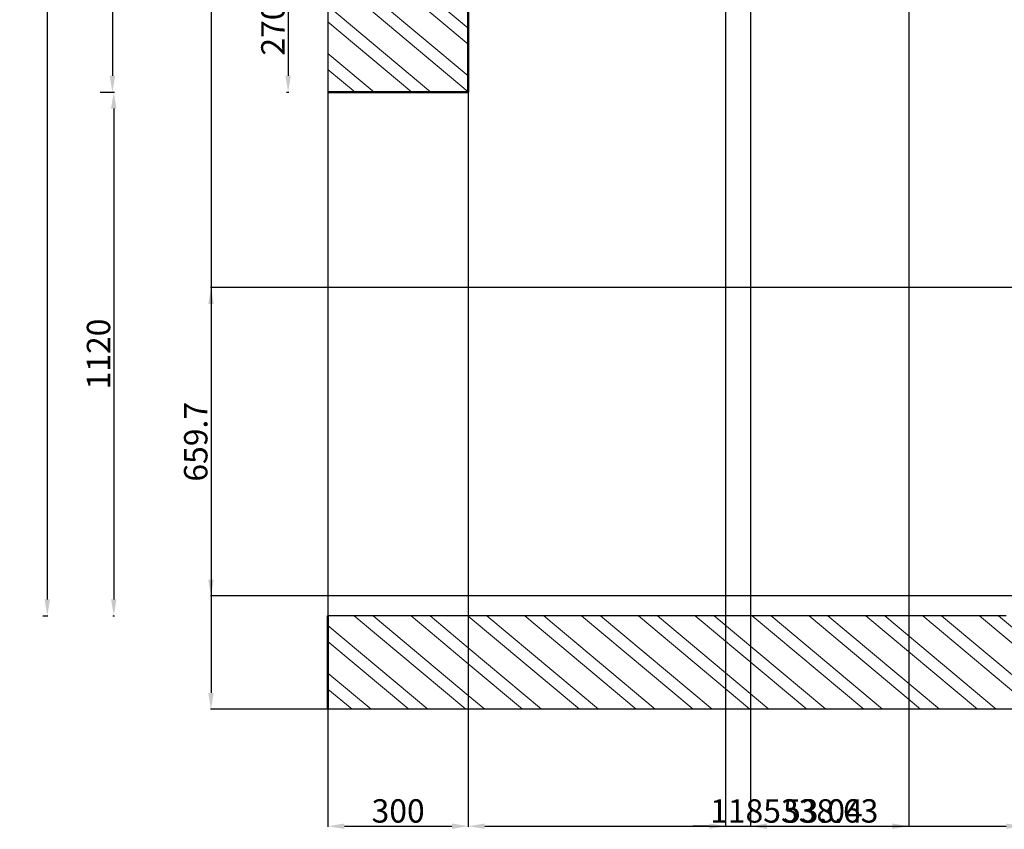
# Model space of a CAD drawing. Units: millimetres. Extents: x 407065 to 421840, y 1168257 to 1177792.
# Tile 3 of 17: x 407065 to 409170, y 1172891 to 1174623. Entities that reach past the tile are written whole.
import ezdxf

# ---------------------------------------------------------------- set-up
doc = ezdxf.new("R2010")
doc.units = ezdxf.units.MM
doc.linetypes.add('DASHED', pattern=[19.05, 12.7, -6.35])
for name, color, linetype, lineweight in [('A-ANNO-DIMS', 6, 'Continuous', 18), ('A-FURN', 3, 'Continuous', 25), ('A-FURN-HIDN', 7, 'DASHED', 18), ('A-WALL', 7, 'Continuous', 50), ('A-WALL-PATT', 8, 'Continuous', 13)]:
    doc.layers.add(name, color=color, linetype=linetype, lineweight=lineweight)
doc.styles.get("Standard").update_dxf_attribs({"font": 'arial.ttf'})
doc.dimstyles.new('ISO-25', dxfattribs={"dimtxt": 50, "dimasz": 35, "dimexe": 1.25, "dimexo": 0.625, "dimtad": 1, "dimdec": 1, "dimtxsty": 'Standard', "dimcen": 35, "dimadec": 0, "dimazin": 0, "dimtfac": 1, "dimtdec": 1, "dimtmove": 0, "dimatfit": 3, "dimfxl": 1, "dimarcsym": 0})

# ---------------------------------------------------------------- blocks, each defined once
blk = doc.blocks.new('*D43')
at = {"layer": 'A-ANNO-DIMS', "color": 0, "lineweight": -2, "transparency": 16777216}
for p, q in [((407635.4, 1174737.8), (407640.4, 1174737.8)), ((407639.2, 1174702.8), (407639.2, 1174502.8)), ((407635.4, 1174467.8), (407640.4, 1174467.8))]:
    blk.add_line(p, q, dxfattribs=at)
at = {"layer": 'A-ANNO-DIMS', "color": 0, "transparency": 16777216}
for points in [[(407633.3, 1174702.8), (407645, 1174702.8), (407639.2, 1174737.8)], [(407633.3, 1174502.8), (407645, 1174502.8), (407639.2, 1174467.8)]]:
    blk.add_solid(points, dxfattribs=at)
at = {"layer": 'Defpoints', "color": 0, "transparency": 16777216}
for p in [(407634.8, 1174737.8), (407634.8, 1174467.8), (407639.2, 1174467.8)]:
    blk.add_point(p, dxfattribs=at)
at = {"layer": 'A-ANNO-DIMS', "color": 0, "transparency": 16777216, "insert": (407613, 1174602.8), "char_height": 50, "attachment_point": 5, "rotation": 90}
blk.add_mtext('270', dxfattribs=at)
blk = doc.blocks.new('*D50')
at = {"layer": 'A-ANNO-DIMS', "color": 0, "lineweight": -2, "transparency": 16777216}
for p, q in [((407237.7, 1177137.8), (407264.8, 1177137.8)), ((407263.5, 1177102.8), (407263.5, 1174502.8)), ((407237.7, 1174467.8), (407264.8, 1174467.8))]:
    blk.add_line(p, q, dxfattribs=at)
at = {"layer": 'A-ANNO-DIMS', "color": 0, "transparency": 16777216}
for points in [[(407257.7, 1177102.8), (407269.4, 1177102.8), (407263.5, 1177137.8)], [(407257.7, 1174502.8), (407269.4, 1174502.8), (407263.5, 1174467.8)]]:
    blk.add_solid(points, dxfattribs=at)
at = {"layer": 'Defpoints', "color": 0, "transparency": 16777216}
for p in [(407237, 1177137.8), (407237, 1174467.8), (407263.5, 1174467.8)]:
    blk.add_point(p, dxfattribs=at)
at = {"layer": 'A-ANNO-DIMS', "color": 0, "transparency": 16777216, "insert": (407237.4, 1175802.8), "char_height": 50, "attachment_point": 5, "rotation": 90}
blk.add_mtext('2670', dxfattribs=at)
blk = doc.blocks.new('*D51')
at = {"layer": 'A-ANNO-DIMS', "color": 0, "lineweight": -2, "transparency": 16777216}
for p, q in [((407115, 1177137.8), (407125.6, 1177137.8)), ((407124.3, 1177102.8), (407124.3, 1173382.8)), ((407115, 1173347.8), (407125.6, 1173347.8))]:
    blk.add_line(p, q, dxfattribs=at)
at = {"layer": 'A-ANNO-DIMS', "color": 0, "transparency": 16777216}
for points in [[(407118.5, 1177102.8), (407130.2, 1177102.8), (407124.3, 1177137.8)], [(407118.5, 1173382.8), (407130.2, 1173382.8), (407124.3, 1173347.8)]]:
    blk.add_solid(points, dxfattribs=at)
at = {"layer": 'Defpoints', "color": 0, "transparency": 16777216}
for p in [(407114.4, 1177137.8), (407114.4, 1173347.8), (407124.3, 1173347.8)]:
    blk.add_point(p, dxfattribs=at)
at = {"layer": 'A-ANNO-DIMS', "color": 0, "transparency": 16777216, "insert": (407098.2, 1175242.8), "char_height": 50, "attachment_point": 5, "rotation": 90}
blk.add_mtext('3790', dxfattribs=at)
blk = doc.blocks.new('*D52')
at = {"layer": 'A-ANNO-DIMS', "color": 0, "lineweight": -2, "transparency": 16777216}
for p, q in [((407264.2, 1174467.8), (407267.7, 1174467.8)), ((407266.5, 1174432.8), (407266.5, 1173382.8)), ((407264.2, 1173347.8), (407267.7, 1173347.8))]:
    blk.add_line(p, q, dxfattribs=at)
at = {"layer": 'A-ANNO-DIMS', "color": 0, "transparency": 16777216}
for points in [[(407260.6, 1174432.8), (407272.3, 1174432.8), (407266.5, 1174467.8)], [(407260.6, 1173382.8), (407272.3, 1173382.8), (407266.5, 1173347.8)]]:
    blk.add_solid(points, dxfattribs=at)
at = {"layer": 'Defpoints', "color": 0, "transparency": 16777216}
for p in [(407263.5, 1174467.8), (407263.5, 1173347.8), (407266.5, 1173347.8)]:
    blk.add_point(p, dxfattribs=at)
at = {"layer": 'A-ANNO-DIMS', "color": 0, "transparency": 16777216, "insert": (407240.3, 1173907.8), "char_height": 50, "attachment_point": 5, "rotation": 90}
blk.add_mtext('1120', dxfattribs=at)
blk = doc.blocks.new('*D166')
at = {"layer": 'A-ANNO-DIMS', "color": 0, "lineweight": -2, "transparency": 16777216}
for p, q in [((407723.7, 1177437.8), (407473.1, 1177437.8)), ((407474.3, 1177402.8), (407474.3, 1173182.8)), ((407723.7, 1173147.8), (407473.1, 1173147.8))]:
    blk.add_line(p, q, dxfattribs=at)
at = {"layer": 'A-ANNO-DIMS', "color": 0, "transparency": 16777216}
for points in [[(407468.5, 1177402.8), (407480.1, 1177402.8), (407474.3, 1177437.8)], [(407468.5, 1173182.8), (407480.1, 1173182.8), (407474.3, 1173147.8)]]:
    blk.add_solid(points, dxfattribs=at)
at = {"layer": 'Defpoints', "color": 0, "transparency": 16777216}
for p in [(407724.3, 1177437.8), (407474.3, 1173147.8), (407724.3, 1173147.8)]:
    blk.add_point(p, dxfattribs=at)
at = {"layer": 'A-ANNO-DIMS', "color": 0, "transparency": 16777216, "insert": (407448.2, 1175292.8), "char_height": 50, "attachment_point": 5, "rotation": 90}
blk.add_mtext('4290', dxfattribs=at)
blk = doc.blocks.new('*D167')
at = {"layer": 'A-ANNO-DIMS', "color": 0, "lineweight": -2, "transparency": 16777216}
for p, q in [((407724.3, 1174467.2), (407724.3, 1172896.5)), ((408024.3, 1174467.2), (408024.3, 1172896.5)), ((407759.3, 1172897.8), (407989.3, 1172897.8))]:
    blk.add_line(p, q, dxfattribs=at)
at = {"layer": 'A-ANNO-DIMS', "color": 0, "transparency": 16777216}
for points in [[(407759.3, 1172903.6), (407759.3, 1172892), (407724.3, 1172897.8)], [(407989.3, 1172903.6), (407989.3, 1172892), (408024.3, 1172897.8)]]:
    blk.add_solid(points, dxfattribs=at)
at = {"layer": 'Defpoints', "color": 0, "transparency": 16777216}
for p in [(407724.3, 1174467.8), (408024.3, 1174467.8), (408024.3, 1172897.8)]:
    blk.add_point(p, dxfattribs=at)
at = {"layer": 'A-ANNO-DIMS', "color": 0, "transparency": 16777216, "insert": (407874.3, 1172924), "char_height": 50, "attachment_point": 5}
blk.add_mtext('300', dxfattribs=at)
blk = doc.blocks.new('*D174')
at = {"layer": 'A-ANNO-DIMS', "color": 0, "lineweight": -2, "transparency": 16777216}
for p, q in [((408627.4, 1176861), (408627.4, 1172896.5)), ((408966, 1176861), (408966, 1172896.5)), ((408662.4, 1172897.8), (408931, 1172897.8))]:
    blk.add_line(p, q, dxfattribs=at)
at = {"layer": 'A-ANNO-DIMS', "color": 0, "transparency": 16777216}
for points in [[(408662.4, 1172903.6), (408662.4, 1172892), (408627.4, 1172897.8)], [(408931, 1172903.6), (408931, 1172892), (408966, 1172897.8)]]:
    blk.add_solid(points, dxfattribs=at)
at = {"layer": 'Defpoints', "color": 0, "transparency": 16777216}
for p in [(408627.4, 1176861.7), (408966, 1176861.7), (408966, 1172897.8)]:
    blk.add_point(p, dxfattribs=at)
at = {"layer": 'A-ANNO-DIMS', "color": 0, "transparency": 16777216, "insert": (408796.7, 1172924), "char_height": 50, "attachment_point": 5}
blk.add_mtext('338.63', dxfattribs=at)
blk = doc.blocks.new('*D176')
at = {"layer": 'A-ANNO-DIMS', "color": 0, "lineweight": -2, "transparency": 16777216}
for p, q in [((408574.3, 1176984.8), (408574.3, 1172896.5)), ((408627.4, 1176861), (408627.4, 1172896.5)), ((408539.3, 1172897.8), (408504.3, 1172897.8)), ((408574.3, 1172897.8), (408627.4, 1172897.8)), ((408662.4, 1172897.8), (408867.1, 1172897.8))]:
    blk.add_line(p, q, dxfattribs=at)
at = {"layer": 'A-ANNO-DIMS', "color": 0, "transparency": 16777216}
for points in [[(408539.3, 1172903.6), (408539.3, 1172892), (408574.3, 1172897.8)], [(408662.4, 1172903.6), (408662.4, 1172892), (408627.4, 1172897.8)]]:
    blk.add_solid(points, dxfattribs=at)
at = {"layer": 'Defpoints', "color": 0, "transparency": 16777216}
for p in [(408574.3, 1176985.5), (408627.4, 1176861.7), (408627.4, 1172897.8)]:
    blk.add_point(p, dxfattribs=at)
at = {"layer": 'A-ANNO-DIMS', "color": 0, "transparency": 16777216, "insert": (408782.2, 1172924), "char_height": 50, "attachment_point": 5}
blk.add_mtext('53.04', dxfattribs=at)
blk = doc.blocks.new('*D187')
at = {"layer": 'A-ANNO-DIMS', "color": 0, "lineweight": -2, "transparency": 16777216}
for p, q in [((409263.3, 1174049.9), (407473.1, 1174049.9)), ((407474.3, 1174014.9), (407474.3, 1173425.2)), ((409263.3, 1173390.2), (407473.1, 1173390.2))]:
    blk.add_line(p, q, dxfattribs=at)
at = {"layer": 'A-ANNO-DIMS', "color": 0, "transparency": 16777216}
for points in [[(407468.5, 1174014.9), (407480.1, 1174014.9), (407474.3, 1174049.9)], [(407468.5, 1173425.2), (407480.1, 1173425.2), (407474.3, 1173390.2)]]:
    blk.add_solid(points, dxfattribs=at)
at = {"layer": 'Defpoints', "color": 0, "transparency": 16777216}
for p in [(409263.9, 1174049.9), (407474.3, 1173390.2), (409263.9, 1173390.2)]:
    blk.add_point(p, dxfattribs=at)
at = {"layer": 'A-ANNO-DIMS', "color": 0, "transparency": 16777216, "insert": (407448.2, 1173720), "char_height": 50, "attachment_point": 5, "rotation": 90}
blk.add_mtext('659.7', dxfattribs=at)
blk = doc.blocks.new('*D188')
at = {"layer": 'A-ANNO-DIMS', "color": 0, "lineweight": -2, "transparency": 16777216}
for p, q in [((408024.3, 1174467.2), (408024.3, 1172896.5)), ((409209.2, 1173444.3), (409209.2, 1172896.5)), ((408059.3, 1172897.8), (409174.2, 1172897.8))]:
    blk.add_line(p, q, dxfattribs=at)
at = {"layer": 'A-ANNO-DIMS', "color": 0, "transparency": 16777216}
for points in [[(408059.3, 1172903.6), (408059.3, 1172892), (408024.3, 1172897.8)], [(409174.2, 1172903.6), (409174.2, 1172892), (409209.2, 1172897.8)]]:
    blk.add_solid(points, dxfattribs=at)
at = {"layer": 'Defpoints', "color": 0, "transparency": 16777216}
for p in [(408024.3, 1174467.8), (409209.2, 1173444.9), (409209.2, 1172897.8)]:
    blk.add_point(p, dxfattribs=at)
at = {"layer": 'A-ANNO-DIMS', "color": 0, "transparency": 16777216, "insert": (408616.8, 1172923.9), "char_height": 50, "attachment_point": 5}
blk.add_mtext('1185', dxfattribs=at)

msp = doc.modelspace()

# ---------------------------------------------------------------- hatches: boundary and pattern name
at = {"layer": 'A-WALL-PATT'}
h = msp.add_hatch(dxfattribs=at)
h.set_pattern_fill('ANSI32', color=256, scale=8.2, angle=95)
h.paths.add_polyline_path([(408024.3133, 1177137.7952), (407724.3133, 1177137.7952), (407724.3133, 1174467.7952), (408024.3133, 1174467.7952)])
h = msp.add_hatch(dxfattribs=at)
h.set_pattern_fill('ANSI32', color=256, scale=8.2, angle=95)
h.paths.add_polyline_path([(408024.3133, 1173347.7952), (407724.3133, 1173347.7952), (407724.3133, 1173147.7952), (408024.3133, 1173147.7952)])
h = msp.add_hatch(dxfattribs=at)
h.set_pattern_fill('ANSI32', color=256, scale=8.2, angle=95)
h.paths.add_polyline_path([(411024.3133, 1173347.7952), (409174.3133, 1173347.7952), (408024.3133, 1173347.7952), (408024.3133, 1173147.7952), (411024.3133, 1173147.7952)])

# ---------------------------------------------------------------- linework, layer by layer
at = {"layer": 'A-FURN'}
for p, q in [((407724.3133, 1177437.7952), (407724.3133, 1174467.7952)), ((409174.3133, 1173347.7952), (407724.3133, 1173347.7952)), ((411024.3133, 1173147.7952), (407724.3133, 1173147.7952))]:
    msp.add_line(p, q, dxfattribs=at)
at = {"layer": 'A-FURN-HIDN'}
for p, q in [((407724.3133, 1174467.7952), (407724.3133, 1173347.7952)), ((408024.3133, 1174467.7952), (408024.3133, 1173147.7952))]:
    msp.add_line(p, q, dxfattribs=at)
at = {"layer": 'A-WALL'}
for p, q in [((408024.3133, 1177137.7952), (408024.3133, 1174467.7952)), ((408024.3133, 1174467.7952), (407724.3133, 1174467.7952)), ((407724.3133, 1173347.7952), (407724.3133, 1173147.7952))]:
    msp.add_line(p, q, dxfattribs=at)

# ---------------------------------------------------------------- dimensions: what is measured, and where the dimension line sits
at = {"layer": 'A-ANNO-DIMS'}
for base, p1, p2, override, picture, middle in [((407474.3133, 1173147.7952), (407724.3133, 1177437.7952), (407724.3133, 1173147.7952), {"dimdec": 0, "dimlfac": 1, "dimrnd": 0, "dimzin": 0, "dimdsep": 46, "dimlunit": 2}, '*D166', (407448.1597, 1175292.7952)), ((407124.3456, 1173347.7952), (407114.4021, 1177137.7952), (407114.4021, 1173347.7952), {"dimclrd": 0, "dimclre": 0, "dimclrt": 0}, '*D51', (407098.1749, 1175242.7952)), ((407263.5498, 1174467.7952), (407237.0345, 1177137.7952), (407237.0345, 1174467.7952), {"dimclrd": 0, "dimclre": 0, "dimclrt": 0}, '*D50', (407237.3961, 1175802.7952)), ((407639.152, 1174467.7952), (407634.777, 1174737.7952), (407634.777, 1174467.7952), {"dimclrd": 0, "dimclre": 0, "dimclrt": 0}, '*D43', (407612.9983, 1174602.7952)), ((407266.4664, 1173347.7952), (407263.5498, 1174467.7952), (407263.5498, 1173347.7952), {"dimclrd": 0, "dimclre": 0, "dimclrt": 0}, '*D52', (407240.3128, 1173907.7952)), ((407474.3133, 1173390.1772), (409263.9371, 1174049.9098), (409263.9371, 1173390.1772), {"dimdec": 1, "dimlfac": 1, "dimrnd": 0, "dimzin": 0, "dimdsep": 46, "dimlunit": 2}, '*D187', (407448.1597, 1173720.0435))]:
    dim = msp.add_linear_dim(base=base, p1=p1, p2=p2, angle=90, dimstyle='ISO-25', override=override, dxfattribs=at)
    dim.commit()
    dim.dimension.update_dxf_attribs({"geometry": picture, "text_midpoint": middle})
for base, p1, p2, override, picture, middle in [((408627.3554, 1172897.7952), (408574.3133, 1176985.4747), (408627.3554, 1176861.6588), {"dimdec": 2, "dimlfac": 1, "dimrnd": 0, "dimzin": 0, "dimdsep": 46, "dimlunit": 2}, '*D176', (408782.2403, 1172923.9659)), ((408965.99043, 1172897.79525), (408627.35545, 1176861.65877), (408965.99043, 1176861.65877), {"dimdec": 2, "dimlfac": 1, "dimrnd": 0, "dimzin": 0, "dimdsep": 46, "dimlunit": 2}, '*D174', (408796.67294, 1172923.96595)), ((408024.3133, 1172897.7952), (407724.3133, 1174467.7952), (408024.3133, 1174467.7952), {"dimdec": 0, "dimlfac": 1, "dimrnd": 0, "dimzin": 0, "dimdsep": 46, "dimlunit": 2}, '*D167', (407874.3133, 1172923.9659)), ((409209.2087, 1172897.7952), (408024.3133, 1174467.7952), (409209.2087, 1173444.9056), {"dimdec": 0, "dimlfac": 1, "dimrnd": 0, "dimzin": 0, "dimdsep": 46, "dimlunit": 2}, '*D188', (408616.761, 1172923.9489))]:
    dim = msp.add_linear_dim(base=base, p1=p1, p2=p2, dimstyle='ISO-25', override=override, dxfattribs=at)
    dim.commit()
    dim.dimension.update_dxf_attribs({"geometry": picture, "text_midpoint": middle})

doc.saveas('drawing.dxf')
